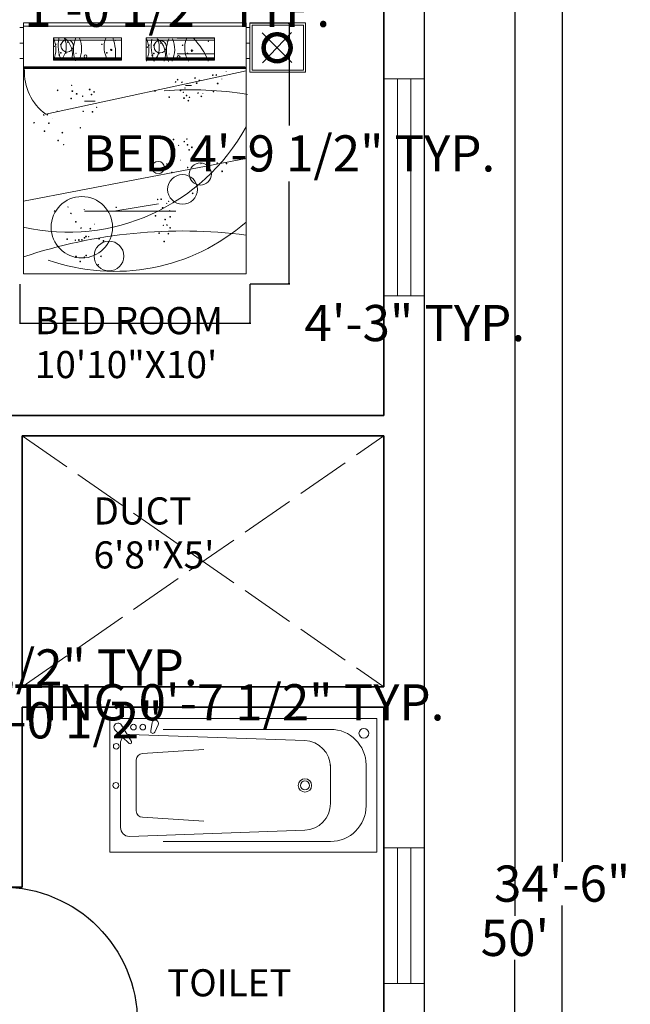
# Model space of a CAD drawing. Units: inches. Extents: x -11 to 443, y 65 to 743.
# Tile 9 of 10: x 243 to 378, y 392 to 610. Entities that reach past the tile are written whole.
import ezdxf

# ---------------------------------------------------------------- set-up
doc = ezdxf.new("R2010")
doc.units = ezdxf.units.IN
doc.header["$MEASUREMENT"] = 0
doc.linetypes.add('ACAD_ISO02W100', pattern=[15, 12, -3])
for name, color, linetype, lineweight in [('A-ANNO-DIMS', 2, 'Continuous', 18), ('A-AREA-IDEN', 2, 'Continuous', 18), ('A-DOOR', 4, 'Continuous', 25), ('A-FLOR-FIXT', 8, 'Continuous', 18), ('A-FLOR-VOID', 8, 'ACAD_ISO02W100', 13), ('A-FURN-PATT', 8, 'Continuous', 9), ('A-GLAZ', 4, 'Continuous', 18), ('A-WALL', 7, 'Continuous', 35), ('C-PROP', 3, 'Continuous', 30), ('Furniture', 7, 'Continuous', 15)]:
    doc.layers.add(name, color=color, linetype=linetype, lineweight=lineweight)
doc.styles.get("Standard").update_dxf_attribs({"font": 'italic8.shx'})
doc.dimstyles.get("Standard").update_dxf_attribs({"dimtxt": 8, "dimasz": 0.18, "dimexe": 0.18, "dimexo": 0.0625, "dimgap": 0.09, "dimtad": 0, "dimtih": 1, "dimtoh": 1, "dimzin": 0, "dimdsep": 46, "dimlunit": 3, "dimtxsty": 'Standard', "dimblk": 'CLOSEDBLANK', "dimcen": 0.09, "dimclrd": 6, "dimclre": 5, "dimclrt": 4, "dimadec": 0, "dimazin": 0, "dimtfac": 1, "dimtofl": 0, "dimtmove": 0, "dimatfit": 3, "dimfxl": 1, "dimtolj": 1, "dimtzin": 0, "dimarcsym": 0})

# ---------------------------------------------------------------- blocks, each defined once
blk = doc.blocks.new('_ClosedBlank')
at = {"color": 0, "linetype": 'ByBlock', "lineweight": -2}
for p, q in [((-1, 0.167), (0, 0)), ((-1, 0.167), (-1, -0.167)), ((0, 0), (-1, -0.167))]:
    blk.add_line(p, q, dxfattribs=at)
blk = doc.blocks.new('*D6')
at = {"layer": 'A-ANNO-DIMS', "color": 0, "lineweight": -2, "transparency": 16777216}
for p, q in [((332.27, 706.92), (352.4, 706.92)), ((352.22, 706.74), (352.22, 411.77)), ((352.22, 107.1), (352.22, 402.07)), ((332.27, 106.92), (352.4, 106.92))]:
    blk.add_line(p, q, dxfattribs=at)
at = {"layer": 'Defpoints', "color": 0, "lineweight": 100, "transparency": 16777216}
for p in [(332.21, 706.92), (332.21, 106.92), (352.22, 106.92)]:
    blk.add_point(p, dxfattribs=at)
at = {"layer": 'A-ANNO-DIMS', "color": 0, "lineweight": -2, "transparency": 16777216, "xscale": 0.18, "yscale": 0.18, "zscale": 0.18}
for p, rotation in [((352.22, 706.92), 90), ((352.22, 106.92), 270)]:
    blk.add_blockref('_ClosedBlank', p, dxfattribs=dict(at, rotation=rotation))
at = {"layer": 'A-ANNO-DIMS', "color": 0, "transparency": 16777216, "insert": (352.22, 406.92), "char_height": 8, "attachment_point": 5}
blk.add_mtext("\\A1;50'", dxfattribs=at)
blk = doc.blocks.new('DOOR-SWING-30')
for p, q in [((0, 30), (0, 0)), ((2, 29.93), (2, 0)), ((0, 0), (30, 0))]:
    blk.add_line(p, q)
blk.add_arc((0, 0), 30, 0, 90)
blk = doc.blocks.new('WIN-48x9')
for p, q in [((0, 48), (0, 0)), ((9, 48), (0, 48)), ((3, 0), (3, 48)), ((6, 0), (6, 48)), ((9, 0), (9, 48)), ((0, 0), (9, 0))]:
    blk.add_line(p, q)
blk = doc.blocks.new('BED-DOUBLE')
for p, q in [((0.82, 54.51), (0, 54.51)), ((50.12, 55.53), (0.82, 55.53)), ((0.82, 55.53), (0.82, 0)), ((50.12, 54.78), (0.82, 54.78)), ((50.12, 0), (50.12, 55.53)), ((50.12, 0), (50.12, 55.53)), ((50.95, 54.51), (50.12, 54.51)), ((0.82, 51.08), (0, 51.08)), ((7.45, 52.2), (7.45, 47.27)), ((22.51, 52.2), (7.45, 52.2)), ((7.45, 51.71), (22.51, 51.71)), ((22.51, 47.27), (22.51, 52.2)), ((43.08, 52.21), (28.01, 52.21)), ((28.01, 52.21), (28.01, 47.28)), ((28.01, 51.71), (43.1, 51.71)), ((43.08, 52.14), (34.85, 52.14)), ((43.08, 47.28), (43.08, 52.21)), ((50.95, 51.08), (50.12, 51.08)), ((43.08, 48.66), (34.85, 48.66)), ((0.82, 47.66), (0, 47.66)), ((0.82, 45.79), (49.9, 45.79)), ((7.45, 47.77), (22.51, 47.77)), ((7.45, 47.56), (22.51, 47.56)), ((7.45, 47.35), (22.51, 47.35)), ((7.45, 47.27), (22.51, 47.27)), ((28.01, 47.77), (43.1, 47.77)), ((28.01, 47.56), (43.1, 47.56)), ((28.01, 47.35), (43.1, 47.35)), ((28.01, 47.28), (43.08, 47.28)), ((50.95, 47.66), (50.12, 47.66)), ((0.81, 45.69), (50.11, 45.69)), ((0.81, 45.48), (50.11, 45.48)), ((5.76, 35.31), (50.13, 44.94)), ((38, 41.71), (36.72, 41.71)), ((16.71, 38.23), (14.33, 38.23)), ((0.81, 16.07), (50.11, 25.52)), ((30.69, 15.53), (20.82, 13.88)), ((34.54, 13.88), (14.33, 13.88)), ((0.82, 0), (50.12, 0)), ((0.82, 0), (50.12, 0))]:
    blk.add_line(p, q)
for centre, radius in [((7.67, 50.33), 0.0548), ((7.99, 50.77), 0.0548), ((9.09, 50.77), 0.0548), ((10.51, 50.44), 1.37), ((10.62, 51.21), 0.0274), ((10.95, 51.64), 0.0274), ((12.05, 51.64), 0.0274), ((12.05, 50.88), 0.0274), ((18.18, 50.77), 0.0548), ((21.14, 51.64), 0.0274), ((28.25, 50.16), 0.0548), ((28.58, 50.6), 0.0548), ((29.68, 50.6), 0.0548), ((31.1, 50.27), 1.37), ((31.21, 51.03), 0.0274), ((31.53, 51.47), 0.0274), ((32.63, 51.47), 0.0274), ((32.63, 50.71), 0.0274), ((36.03, 50.6), 0.0548), ((41.72, 51.47), 0.0274), ((8.76, 48.47), 0.0822), ((9.09, 48.91), 0.0822), ((10.19, 48.91), 0.0822), ((12.48, 48.8), 0.0274), ((14.56, 48.14), 0.329), ((19.27, 48.91), 0.0822), ((20.26, 49.56), 0.164), ((29.35, 48.3), 0.0822), ((29.67, 48.74), 0.0822), ((30.77, 48.74), 0.0822), ((33.07, 48.63), 0.0274), ((35.15, 47.97), 0.329), ((37.12, 48.74), 0.0822), ((38.11, 49.39), 0.164), ((41.53, 45.6), 0.0822), ((42.72, 43.97), 0.0548), ((43.5, 44.01), 0.0822), ((45.68, 44.84), 0.0274), ((11.51, 41.72), 0.0548), ((34.49, 42.48), 0.0548), ((34.94, 42.97), 0.0822), ((35.9, 42.4), 0.0822), ((38.78, 43.35), 0.0822), ((39.16, 42.2), 0.0822), ((39.74, 42.78), 0.0822), ((43.81, 42.11), 0.0822), ((44.72, 43.1), 0.0274), ((8.39, 40.62), 0.0822), ((11.65, 40.43), 0.0822), ((12.61, 39.86), 0.0822), ((13.92, 39.31), 0.0548), ((15.49, 40.82), 0.0822), ((15.87, 39.67), 0.0822), ((16.44, 40.24), 0.0822), ((29.94, 40.51), 0.0822), ((35.59, 40.62), 0.0822), ((36.22, 40.19), 0.0548), ((36.59, 41.14), 0.0274), ((36.93, 39.48), 0.0822), ((39.48, 40), 0.0548), ((40.19, 39.28), 0.0822), ((40.52, 39.93), 0.0274), ((42.86, 40.37), 0.0822), ((11.37, 38.79), 0.0822), ((33.1, 39.09), 0.0822), ((36.35, 38.9), 0.0822), ((37.31, 38.33), 0.0822), ((37.56, 39.06), 0.0548), ((5.33, 35.19), 0.0548), ((6.11, 35.23), 0.0822), ((8.29, 36.06), 0.0274), ((14.06, 35.98), 0.0548), ((16.11, 35.86), 0.0822), ((17.02, 36.86), 0.0274), ((3.2, 33.44), 0.0548), ((6.43, 33.33), 0.0822), ((7.34, 34.32), 0.0274), ((5.48, 31.58), 0.0822), ((9.44, 31.26), 0.0822), ((13.43, 32.33), 0.0548), ((8.49, 29.52), 0.0822), ((9.72, 28.61), 0.0274), ((33.86, 28.77), 0.0822), ((34.05, 29.73), 0.0822), ((35.15, 28.44), 0.0274), ((36.41, 29.29), 0.0548), ((36.99, 29.87), 0.0548), ((37.12, 28.58), 0.0822), ((34.24, 27.62), 0.0822), ((37.5, 27.43), 0.0822), ((38.08, 28.01), 0.0822), ((30.66, 23.53), 1.37), ((32.57, 24.29), 0.0548), ((33.81, 25.44), 0.0274), ((35.53, 25.17), 0.0274), ((39.97, 22.1), 2.46), ((40.13, 24.42), 0.0274), ((43.71, 24.56), 0.0548), ((45.75, 24.45), 0.0822), ((36.03, 18.71), 3.29), ((33.67, 22.43), 0.0822), ((37.18, 23.55), 0.0548), ((44.8, 22.7), 0.0822), ((38.27, 17.83), 0.0822), ((13.75, 10.33), 6.79), ((30.53, 16.48), 0.0548), ((31.31, 16.52), 0.0822), ((32.54, 15.61), 0.0274), ((32.96, 16.06), 0.0548), ((7.71, 13.94), 0.0548), ((10.67, 14.82), 0.0274), ((11.32, 13.38), 0.0548), ((14.28, 14.25), 0.0274), ((21.36, 14.74), 0.0548), ((31.63, 14.62), 0.0822), ((33.15, 13.95), 0.0548), ((12.42, 11.52), 0.0822), ((16.54, 11.02), 0.0274), ((30.03, 12.86), 0.0822), ((32.19, 12.04), 0.0548), ((32.58, 10.82), 0.0822), ((33.29, 12.66), 0.0822), ((13.59, 10.14), 0.0548), ((15.63, 10.02), 0.0822), ((30.85, 9.03), 0.0548), ((31.8, 10.77), 0.0548), ((32.9, 8.91), 0.0822), ((33.29, 10.18), 0.0822), ((10.5, 7.72), 0.0822), ((12.32, 7.47), 0.0548), ((13.09, 7.51), 0.0822), ((13.76, 7.53), 0.0822), ((14.33, 8.01), 0.0822), ((14.68, 8.28), 0.0822), ((15.27, 8.25), 0.0274), ((19.76, 3.97), 3.29), ((17.59, 7.82), 0.0822), ((18.55, 7.34), 0.0822), ((31.95, 7.17), 0.0822), ((12.46, 3.87), 0.0822), ((13.41, 2.75), 0.0822), ((14.32, 3.74), 0.0274), ((14.72, 4.1), 0.0822), ((17.98, 3.91), 0.0822), ((17.39, 2.05), 0.0548)]:
    blk.add_circle(centre, radius)
for centre, radius, start, end in [((10.49, 48.64), 10.74, 352.6491, 19.9229), ((2.24, 49.73), 5.76, 334.6876, 25.3124), ((18.3, 50.59), 9.77, 171.2054, 199.8717), ((5.97, 50.26), 4.34, 316.473, 26.5351), ((7.41, 48.73), 4.24, 339.7755, 54.8367), ((18.16, 49.62), 6.28, 155.7867, 203.0598), ((7.63, 49.85), 6.08, 334.8533, 22.5945), ((24.13, 50.16), 5.46, 158.1924, 212.0094), ((22.83, 49.56), 5.76, 334.6876, 25.3124), ((38.89, 50.42), 9.77, 171.2054, 199.8717), ((26.55, 50.09), 4.34, 316.473, 26.5351), ((28, 48.56), 4.24, 339.7755, 54.8367), ((38.74, 49.45), 6.28, 155.7867, 203.0598), ((28.22, 49.68), 6.08, 334.8533, 22.5945), ((41.97, 49.99), 5.46, 158.1924, 212.0094), ((27.71, 41.52), 15.09, 21.7027, 44.6945), ((12.77, 44.72), 11.73, 177.3999, 233.2824), ((37.95, -36.79), 77.52, 80.7462, 94.4176), ((10.65, 54.27), 45.03, 257.3742, 331.1748), ((20.99, 44.94), 44.36, 250.6919, 311.0239), ((35.98, -101.04), 110.55, 82.6585, 108.5509)]:
    blk.add_arc(centre, radius, start, end)
blk = doc.blocks.new('NIGHTSTAND-LAMP')
for p, q in [((0, 10.9), (0, 0)), ((12.32, 10.9), (0, 10.9)), ((12.32, 0), (12.32, 10.9)), ((0.49, 10.41), (0.49, 0.49)), ((11.83, 10.41), (0.49, 10.41)), ((2.81, 2.1), (9.21, 8.77)), ((11.83, 0.49), (11.83, 10.41)), ((2.74, 8.7), (9.27, 2.17)), ((0.49, 0.49), (11.83, 0.49)), ((0, 0), (12.32, 0))]:
    blk.add_line(p, q)
for radius in [3.39, 2.6]:
    blk.add_circle((6.01, 5.43), radius)
blk = doc.blocks.new('*D24')
at = {"layer": 'A-ANNO-DIMS', "color": 5, "lineweight": -2, "transparency": 16777216}
for p, q in [((293.66, 609.27), (302.43, 609.27)), ((293.66, 551.54), (302.43, 551.54))]:
    blk.add_line(p, q, dxfattribs=at)
at = {"layer": 'A-ANNO-DIMS', "color": 6, "lineweight": -2, "transparency": 16777216}
for p, q in [((302.25, 609.09), (302.25, 586.59)), ((302.25, 551.72), (302.25, 574.22))]:
    blk.add_line(p, q, dxfattribs=at)
at = {"layer": 'Defpoints', "color": 0, "lineweight": 100, "transparency": 16777216}
for p in [(293.59, 609.27), (302.25, 609.27), (293.59, 551.54)]:
    blk.add_point(p, dxfattribs=at)
at = {"layer": 'A-ANNO-DIMS', "color": 6, "lineweight": -2, "transparency": 16777216, "xscale": 0.18, "yscale": 0.18, "zscale": 0.18}
for p, rotation in [((302.25, 609.27), 90), ((302.25, 551.54), 270)]:
    blk.add_blockref('_ClosedBlank', p, dxfattribs=dict(at, rotation=rotation))
at = {"layer": 'A-ANNO-DIMS', "color": 4, "transparency": 16777216, "insert": (302.25, 580.41), "char_height": 8, "attachment_point": 5}
blk.add_mtext('\\A1;BED 4\'-9 1/2" TYP.', dxfattribs=at)
blk = doc.blocks.new('*D25')
at = {"layer": 'A-ANNO-DIMS', "color": 5, "lineweight": -2, "transparency": 16777216}
for p, q in [((242.65, 551.48), (242.65, 542.71)), ((293.59, 551.48), (293.59, 542.71))]:
    blk.add_line(p, q, dxfattribs=at)
at = {"layer": 'A-ANNO-DIMS', "color": 6, "lineweight": -2, "transparency": 16777216}
for p, q in [((242.83, 542.89), (293.41, 542.89)), ((293.59, 542.89), (293.77, 542.89))]:
    blk.add_line(p, q, dxfattribs=at)
at = {"layer": 'Defpoints', "color": 0, "lineweight": 100, "transparency": 16777216}
for p in [(242.65, 551.54), (293.59, 551.54), (293.59, 542.89)]:
    blk.add_point(p, dxfattribs=at)
at = {"layer": 'A-ANNO-DIMS', "color": 6, "lineweight": -2, "transparency": 16777216, "xscale": 0.18, "yscale": 0.18, "zscale": 0.18, "rotation": 180}
blk.add_blockref('_ClosedBlank', (242.65, 542.89), dxfattribs=at)
at = {"layer": 'A-ANNO-DIMS', "color": 6, "lineweight": -2, "transparency": 16777216, "xscale": 0.18, "yscale": 0.18, "zscale": 0.18}
blk.add_blockref('_ClosedBlank', (293.59, 542.89), dxfattribs=at)
at = {"layer": 'A-ANNO-DIMS', "color": 4, "transparency": 16777216, "insert": (330.05, 542.89), "char_height": 8, "attachment_point": 5}
blk.add_mtext('\\A1;4\'-3" TYP.', dxfattribs=at)
blk = doc.blocks.new('*D26')
at = {"layer": 'A-ANNO-DIMS', "color": 5, "lineweight": -2, "transparency": 16777216}
for p, q in [((133.01, 610.6), (133.01, 612.57)), ((145.34, 610.6), (145.34, 612.57))]:
    blk.add_line(p, q, dxfattribs=at)
at = {"layer": 'A-ANNO-DIMS', "color": 6, "lineweight": -2, "transparency": 16777216}
for p, q in [((133.19, 612.39), (145.16, 612.39)), ((145.34, 612.39), (145.52, 612.39))]:
    blk.add_line(p, q, dxfattribs=at)
at = {"layer": 'Defpoints', "color": 0, "lineweight": 100, "transparency": 16777216}
for p in [(145.34, 612.39), (133.01, 610.54), (145.34, 610.54)]:
    blk.add_point(p, dxfattribs=at)
at = {"layer": 'A-ANNO-DIMS', "color": 6, "lineweight": -2, "transparency": 16777216, "xscale": 0.18, "yscale": 0.18, "zscale": 0.18, "rotation": 180}
blk.add_blockref('_ClosedBlank', (133.01, 612.39), dxfattribs=at)
at = {"layer": 'A-ANNO-DIMS', "color": 6, "lineweight": -2, "transparency": 16777216, "xscale": 0.18, "yscale": 0.18, "zscale": 0.18}
blk.add_blockref('_ClosedBlank', (145.34, 612.39), dxfattribs=at)
at = {"layer": 'A-ANNO-DIMS', "color": 4, "transparency": 16777216, "insert": (242.18, 612.39), "char_height": 8, "attachment_point": 5}
blk.add_mtext('\\A1;NIGHTSTAND 1\'-0 1/2" TYP.', dxfattribs=at)
blk = doc.blocks.new('*D30')
at = {"layer": 'A-ANNO-DIMS', "color": 5, "lineweight": -2, "transparency": 16777216}
for p, q in [((187.91, 460.07), (187.91, 458.84)), ((195.36, 460.07), (195.36, 458.84))]:
    blk.add_line(p, q, dxfattribs=at)
at = {"layer": 'A-ANNO-DIMS', "color": 6, "lineweight": -2, "transparency": 16777216}
for p, q in [((188.09, 459.02), (195.18, 459.02)), ((195.36, 459.02), (195.54, 459.02))]:
    blk.add_line(p, q, dxfattribs=at)
at = {"layer": 'Defpoints', "color": 0, "lineweight": 100, "transparency": 16777216}
for p in [(187.91, 460.14), (195.36, 460.14), (195.36, 459.02)]:
    blk.add_point(p, dxfattribs=at)
at = {"layer": 'A-ANNO-DIMS', "color": 6, "lineweight": -2, "transparency": 16777216, "xscale": 0.18, "yscale": 0.18, "zscale": 0.18, "rotation": 180}
blk.add_blockref('_ClosedBlank', (187.91, 459.02), dxfattribs=at)
at = {"layer": 'A-ANNO-DIMS', "color": 6, "lineweight": -2, "transparency": 16777216, "xscale": 0.18, "yscale": 0.18, "zscale": 0.18}
blk.add_blockref('_ClosedBlank', (195.36, 459.02), dxfattribs=at)
at = {"layer": 'A-ANNO-DIMS', "color": 4, "transparency": 16777216, "insert": (279.25, 459.02), "char_height": 8, "attachment_point": 5}
blk.add_mtext('\\A1;SETTING 0\'-7 1/2" TYP.', dxfattribs=at)
blk = doc.blocks.new('*D31')
at = {"layer": 'A-ANNO-DIMS', "color": 5, "lineweight": -2, "transparency": 16777216}
for p, q in [((195.43, 466.55), (196.66, 466.55)), ((195.43, 460.14), (196.66, 460.14))]:
    blk.add_line(p, q, dxfattribs=at)
at = {"layer": 'A-ANNO-DIMS', "color": 6, "lineweight": -2, "transparency": 16777216}
for p, q in [((196.48, 466.55), (196.48, 466.73)), ((196.48, 466.73), (196.66, 466.73)), ((196.48, 460.32), (196.48, 466.37))]:
    blk.add_line(p, q, dxfattribs=at)
at = {"layer": 'Defpoints', "color": 0, "lineweight": 100, "transparency": 16777216}
for p in [(195.36, 466.55), (196.48, 466.55), (195.36, 460.14)]:
    blk.add_point(p, dxfattribs=at)
at = {"layer": 'A-ANNO-DIMS', "color": 6, "lineweight": -2, "transparency": 16777216, "xscale": 0.18, "yscale": 0.18, "zscale": 0.18}
for p, rotation in [((196.48, 466.55), 90), ((196.48, 460.14), 270)]:
    blk.add_blockref('_ClosedBlank', p, dxfattribs=dict(at, rotation=rotation))
at = {"layer": 'A-ANNO-DIMS', "color": 4, "transparency": 16777216, "insert": (248.18, 466.73), "char_height": 8, "attachment_point": 5}
blk.add_mtext('\\A1;0\'-6 1/2" TYP.', dxfattribs=at)
blk = doc.blocks.new('*D36')
at = {"layer": 'A-ANNO-DIMS', "color": 5, "lineweight": -2, "transparency": 16777216}
for p, q in [((323.27, 625.92), (362.85, 625.92)), ((323.27, 211.92), (362.85, 211.92))]:
    blk.add_line(p, q, dxfattribs=at)
at = {"layer": 'A-ANNO-DIMS', "color": 6, "lineweight": -2, "transparency": 16777216}
for p, q in [((362.67, 625.74), (362.67, 423.77)), ((362.67, 212.1), (362.67, 414.07))]:
    blk.add_line(p, q, dxfattribs=at)
at = {"layer": 'Defpoints', "color": 0, "lineweight": 100, "transparency": 16777216}
for p in [(323.21, 625.92), (362.67, 625.92), (323.21, 211.92)]:
    blk.add_point(p, dxfattribs=at)
at = {"layer": 'A-ANNO-DIMS', "color": 6, "lineweight": -2, "transparency": 16777216, "xscale": 0.18, "yscale": 0.18, "zscale": 0.18}
for p, rotation in [((362.67, 625.92), 90), ((362.67, 211.92), 270)]:
    blk.add_blockref('_ClosedBlank', p, dxfattribs=dict(at, rotation=rotation))
at = {"layer": 'A-ANNO-DIMS', "color": 4, "transparency": 16777216, "insert": (362.67, 418.92), "char_height": 8, "attachment_point": 5}
blk.add_mtext('\\A1;34\'-6"', dxfattribs=at)
blk = doc.blocks.new('*D41')
at = {"layer": 'A-ANNO-DIMS', "color": 5, "lineweight": -2, "transparency": 16777216}
for p, q in [((191.4, 454.94), (191.4, 455.12)), ((191.31, 455.03), (191.49, 455.03))]:
    blk.add_line(p, q, dxfattribs=at)
at = {"layer": 'A-ANNO-DIMS', "color": 6, "lineweight": -2, "transparency": 16777216}
blk.add_line((210.85, 455.03), (203.74, 455.03), dxfattribs=at)
at = {"layer": 'Defpoints', "color": 0, "lineweight": 100, "transparency": 16777216}
for p in [(179.23, 455.03), (203.56, 455.03)]:
    blk.add_point(p, dxfattribs=at)
at = {"layer": 'A-ANNO-DIMS', "color": 6, "lineweight": -2, "transparency": 16777216, "xscale": 0.18, "yscale": 0.18, "zscale": 0.18, "rotation": 179.9993686908669}
blk.add_blockref('_ClosedBlank', (203.56, 455.03), dxfattribs=at)
at = {"layer": 'A-ANNO-DIMS', "color": 4, "transparency": 16777216, "insert": (247.32, 455.03), "char_height": 8, "attachment_point": 5}
blk.add_mtext('\\A1;∅2\'-0 1/2"', dxfattribs=at)

msp = doc.modelspace()

# ---------------------------------------------------------------- hatches: boundary and pattern name
at = {"layer": 'A-FURN-PATT'}
h = msp.add_hatch(dxfattribs=at)
h.set_pattern_fill('ANSI37', color=256, scale=0.6260848, angle=45, style=0)
h.paths.add_polyline_path([(302.989, 603.779), (302.987, 603.912), (302.979, 604.045), (302.966, 604.177), (302.947, 604.309), (302.924, 604.44), (302.896, 604.57), (302.862, 604.698), (302.823, 604.826), (302.78, 604.951), (302.731, 605.075), (302.678, 605.197), (302.62, 605.317), (302.557, 605.434), (302.49, 605.549), (302.418, 605.661), (302.342, 605.77), (302.262, 605.876), (302.177, 605.979), (302.089, 606.079), (301.997, 606.175), (301.901, 606.267), (301.801, 606.355), (301.699, 606.44), (301.592, 606.52), (301.483, 606.596), (301.371, 606.668), (301.256, 606.735), (301.139, 606.798), (301.019, 606.856), (300.897, 606.909), (300.774, 606.958), (300.648, 607.001), (300.521, 607.04), (300.392, 607.073), (300.262, 607.102), (300.131, 607.125), (299.999, 607.144), (299.867, 607.157), (299.734, 607.164), (299.601, 607.167), (299.468, 607.164), (299.335, 607.157), (299.203, 607.144), (299.071, 607.125), (298.94, 607.102), (298.81, 607.073), (298.681, 607.04), (298.554, 607.001), (298.428, 606.958), (298.304, 606.909), (298.182, 606.856), (298.063, 606.798), (297.945, 606.735), (297.83, 606.668), (297.718, 606.596), (297.609, 606.52), (297.503, 606.44), (297.4, 606.355), (297.301, 606.267), (297.205, 606.175), (297.113, 606.079), (297.024, 605.979), (296.94, 605.876), (296.86, 605.77), (296.784, 605.661), (296.712, 605.549), (296.645, 605.434), (296.582, 605.317), (296.524, 605.197), (296.47, 605.075), (296.422, 604.951), (296.378, 604.826), (296.34, 604.698), (296.306, 604.57), (296.278, 604.44), (296.254, 604.309), (296.236, 604.177), (296.223, 604.045), (296.215, 603.912), (296.213, 603.779), (296.215, 603.646), (296.223, 603.513), (296.236, 603.38), (296.254, 603.249), (296.278, 603.118), (296.306, 602.988), (296.34, 602.859), (296.378, 602.732), (296.422, 602.606), (296.47, 602.482), (296.524, 602.36), (296.582, 602.24), (296.645, 602.123), (296.712, 602.008), (296.784, 601.896), (296.86, 601.787), (296.94, 601.681), (297.024, 601.578), (297.113, 601.479), (297.205, 601.383), (297.301, 601.291), (297.4, 601.202), (297.503, 601.118), (297.609, 601.038), (297.718, 600.961), (297.83, 600.89), (297.945, 600.822), (298.063, 600.76), (298.182, 600.702), (298.304, 600.648), (298.428, 600.6), (298.554, 600.556), (298.681, 600.518), (298.81, 600.484), (298.94, 600.456), (299.071, 600.432), (299.203, 600.414), (299.335, 600.401), (299.468, 600.393), (299.601, 600.39), (299.734, 600.393), (299.867, 600.401), (299.999, 600.414), (300.131, 600.432), (300.262, 600.456), (300.392, 600.484), (300.521, 600.518), (300.648, 600.556), (300.774, 600.6), (300.897, 600.648), (301.019, 600.702), (301.139, 600.76), (301.256, 600.822), (301.371, 600.89), (301.483, 600.961), (301.592, 601.038), (301.699, 601.118), (301.801, 601.202), (301.901, 601.291), (301.997, 601.383), (302.089, 601.479), (302.177, 601.578), (302.262, 601.681), (302.342, 601.787), (302.418, 601.896), (302.49, 602.008), (302.557, 602.123), (302.62, 602.24), (302.678, 602.36), (302.731, 602.482), (302.78, 602.606), (302.823, 602.732), (302.862, 602.859), (302.896, 602.988), (302.924, 603.118), (302.947, 603.249), (302.966, 603.38), (302.979, 603.513), (302.987, 603.646)])
h.paths.add_polyline_path([(302.206, 603.779), (302.204, 603.676), (302.198, 603.574), (302.188, 603.473), (302.174, 603.371), (302.156, 603.271), (302.134, 603.171), (302.108, 603.072), (302.078, 602.974), (302.045, 602.877), (302.007, 602.782), (301.966, 602.688), (301.922, 602.596), (301.874, 602.506), (301.822, 602.418), (301.767, 602.332), (301.708, 602.248), (301.646, 602.166), (301.582, 602.087), (301.514, 602.011), (301.443, 601.937), (301.369, 601.866), (301.293, 601.798), (301.213, 601.733), (301.132, 601.671), (301.048, 601.613), (300.962, 601.558), (300.874, 601.506), (300.783, 601.458), (300.691, 601.413), (300.598, 601.372), (300.502, 601.335), (300.406, 601.301), (300.308, 601.272), (300.209, 601.246), (300.109, 601.224), (300.008, 601.206), (299.907, 601.192), (299.805, 601.182), (299.703, 601.176), (299.601, 601.174), (299.499, 601.176), (299.396, 601.182), (299.295, 601.192), (299.193, 601.206), (299.093, 601.224), (298.993, 601.246), (298.894, 601.272), (298.796, 601.301), (298.699, 601.335), (298.604, 601.372), (298.51, 601.413), (298.418, 601.458), (298.328, 601.506), (298.24, 601.558), (298.154, 601.613), (298.07, 601.671), (297.988, 601.733), (297.909, 601.798), (297.833, 601.866), (297.759, 601.937), (297.688, 602.011), (297.62, 602.087), (297.555, 602.166), (297.494, 602.248), (297.435, 602.332), (297.38, 602.418), (297.328, 602.506), (297.28, 602.596), (297.235, 602.688), (297.194, 602.782), (297.157, 602.877), (297.124, 602.974), (297.094, 603.072), (297.068, 603.171), (297.046, 603.271), (297.028, 603.371), (297.014, 603.473), (297.004, 603.574), (296.998, 603.676), (296.996, 603.779), (296.998, 603.881), (297.004, 603.983), (297.014, 604.085), (297.028, 604.186), (297.046, 604.287), (297.068, 604.387), (297.094, 604.486), (297.124, 604.584), (297.157, 604.68), (297.194, 604.776), (297.235, 604.869), (297.28, 604.961), (297.328, 605.051), (297.38, 605.14), (297.435, 605.226), (297.494, 605.31), (297.555, 605.391), (297.62, 605.47), (297.688, 605.547), (297.759, 605.621), (297.833, 605.691), (297.909, 605.759), (297.988, 605.824), (298.07, 605.886), (298.154, 605.945), (298.24, 606), (298.328, 606.051), (298.418, 606.1), (298.51, 606.144), (298.604, 606.185), (298.699, 606.223), (298.796, 606.256), (298.894, 606.286), (298.993, 606.312), (299.093, 606.333), (299.193, 606.351), (299.295, 606.365), (299.396, 606.376), (299.499, 606.382), (299.601, 606.384), (299.703, 606.382), (299.805, 606.376), (299.907, 606.365), (300.008, 606.351), (300.109, 606.333), (300.209, 606.312), (300.308, 606.286), (300.406, 606.256), (300.502, 606.223), (300.598, 606.185), (300.691, 606.144), (300.783, 606.1), (300.874, 606.051), (300.962, 606), (301.048, 605.945), (301.132, 605.886), (301.213, 605.824), (301.293, 605.759), (301.369, 605.691), (301.443, 605.621), (301.514, 605.547), (301.582, 605.47), (301.646, 605.391), (301.708, 605.31), (301.767, 605.226), (301.822, 605.14), (301.874, 605.051), (301.922, 604.961), (301.966, 604.869), (302.007, 604.776), (302.045, 604.68), (302.078, 604.584), (302.108, 604.486), (302.134, 604.387), (302.156, 604.287), (302.174, 604.186), (302.188, 604.085), (302.198, 603.983), (302.204, 603.881)], flags=0)

# ---------------------------------------------------------------- linework, layer by layer
at = {"layer": 'A-FLOR-FIXT'}
for p, q in [((321.647, 455.401), (262.592, 455.401)), ((262.592, 455.401), (262.592, 425.874)), ((321.647, 425.874), (321.647, 455.401)), ((267.374, 450.325), (265.186, 453.955)), ((271.942, 454.519), (271.636, 452.692)), ((272.529, 452.413), (273.292, 454.034)), ((311.411, 453.039), (274.403, 453.039)), ((263.744, 452.888), (266.889, 449.933)), ((266.923, 451.912), (305.712, 450.556)), ((264.954, 449.944), (264.954, 431.331)), ((269.823, 447.665), (283.355, 448.561)), ((268.445, 446.287), (268.445, 434.988)), ((311.411, 436.62), (311.411, 445.165)), ((319.285, 436.11), (319.285, 445.165)), ((269.823, 433.61), (283.355, 432.714)), ((266.923, 429.363), (305.712, 430.718)), ((274.403, 428.236), (311.411, 428.236)), ((262.592, 425.874), (321.647, 425.874))]:
    msp.add_line(p, q, dxfattribs=at)
for centre, radius in [((267.818, 453.531), 0.628), ((269.883, 453.531), 0.628), ((318.797, 452.162), 1.086), ((264.013, 449.286), 0.628), ((305.767, 440.637), 1.476), ((263.934, 440.637), 0.656), ((305.767, 440.637), 0.984)]:
    msp.add_circle(centre, radius, dxfattribs=at)
for centre, radius, start, end in [((264.404, 453.504), 0.903, 29.98081, 223.02252), ((272.644, 454.354), 0.722, 333.70215, 166.74386), ((311.411, 445.165), 7.874, 0, 90), ((266.923, 449.944), 1.968, 137.68629, 180), ((266.923, 449.944), 1.968, 137.68629, 180), ((266.923, 449.944), 1.968, 90, 103.84203), ((266.923, 449.944), 1.968, 90, 103.84203), ((272.102, 452.614), 0.472, 170.49628, 334.80018), ((267.105, 450.162), 0.315, 226.77494, 31.07884), ((267.105, 450.162), 0.315, 226.77494, 31.07884), ((305.506, 444.655), 5.905, 0, 87.99837), ((269.823, 446.287), 1.378, 90, 180), ((305.506, 436.62), 5.905, 272.00163, 0), ((311.411, 436.11), 7.874, 270, 0), ((269.823, 434.988), 1.378, 180, 270), ((266.923, 431.331), 1.968, 180, 270)]:
    msp.add_arc(centre, radius, start, end, dxfattribs=at)
at = {"layer": 'A-FLOR-VOID'}
for p, q in [((243.209, 462.42), (323.209, 517.92)), ((243.209, 517.92), (323.209, 462.42))]:
    msp.add_line(p, q, dxfattribs=at)
at = {"layer": 'A-GLAZ'}
for p, q in [((323.209, 396.826), (323.209, 426.826)), ((323.209, 426.826), (332.209, 426.826)), ((326.209, 426.826), (326.209, 396.826)), ((329.209, 426.826), (329.209, 396.826)), ((332.209, 426.826), (332.209, 396.826)), ((332.209, 396.826), (323.209, 396.826))]:
    msp.add_line(p, q, dxfattribs=at)
at = {"layer": 'A-WALL'}
for p, q in [((323.209, 522.42), (323.209, 616.92)), ((236.859, 522.42), (323.209, 522.42)), ((243.209, 517.92), (323.209, 517.92)), ((243.209, 462.42), (243.209, 517.92)), ((323.209, 462.42), (323.209, 517.92)), ((243.209, 462.42), (323.209, 462.42)), ((243.209, 457.92), (323.209, 457.92)), ((243.209, 418.17), (243.209, 457.92)), ((323.209, 378.42), (323.209, 457.92)), ((243.209, 418.17), (238.709, 418.17))]:
    msp.add_line(p, q, dxfattribs=at)
at = {"layer": 'C-PROP'}
msp.add_lwpolyline([(44.209, 106.92), (332.209, 106.92), (332.209, 706.92), (44.209, 706.92)], close=True, dxfattribs=at)

# ---------------------------------------------------------------- block references
at = {"layer": 'A-DOOR', "extrusion": (0, 0, -1), "zscale": -1, "rotation": 90.00000000000003}
msp.add_blockref('DOOR-SWING-30', (-238.709, 388.169), dxfattribs=at)
at = {"layer": 'A-GLAZ'}
msp.add_blockref('WIN-48x9', (323.209, 548.882), dxfattribs=at)
at = {"layer": 'Furniture'}
for name, p in [('BED-DOUBLE', (242.648, 553.738)), ('NIGHTSTAND-LAMP', (293.594, 598.345))]:
    msp.add_blockref(name, p, dxfattribs=at)

# ---------------------------------------------------------------- texts
at = {"layer": 'A-AREA-IDEN'}
for s, p in [('BED ROOM', (245.989, 540.418)), ('10\'10"X10\'', (245.989, 530.704)), ('DUCT', (258.989, 498.336)), ('6\'8"X5\'', (258.989, 488.622)), ('TOILET', (275.264, 393.986))]:
    msp.add_text(s, height=6, dxfattribs=at).set_placement(p)

# ---------------------------------------------------------------- dimensions: what is measured, and where the dimension line sits
at = {"layer": 'A-ANNO-DIMS'}
for base, p1, p2, override, picture, middle in [((352.221, 106.92), (332.209, 706.92), (332.209, 106.92), {"dimclrd": 0, "dimclre": 0, "dimclrt": 0}, '*D6', (352.221, 406.92)), ((362.669, 625.92), (323.209, 211.92), (323.209, 625.92), {"dimdec": 1, "dimlfac": 1, "dimrnd": 0, "dimzin": 1, "dimdsep": 46, "dimlunit": 4, "dimfrac": 2}, '*D36', (362.669, 418.92))]:
    dim = msp.add_linear_dim(base=base, p1=p1, p2=p2, angle=90, dimstyle='Standard', override=override, dxfattribs=at)
    dim.commit()
    dim.dimension.update_dxf_attribs({"geometry": picture, "text_midpoint": middle})
for base, p1, p2, text, picture, middle in [((145.337, 612.387), (133.013, 610.539), (145.337, 610.539), 'NIGHTSTAND <> TYP.', '*D26', (242.179, 612.387)), ((293.593, 542.886), (242.648, 551.544), (293.593, 551.544), '<> TYP.', '*D25', (330.054, 542.886)), ((195.365, 459.019), (187.912, 460.137), (195.365, 460.137), 'SETTING <> TYP.', '*D30', (279.254, 459.019))]:
    dim = msp.add_linear_dim(base=base, p1=p1, p2=p2, text=text, dimstyle='Standard', override={"dimdec": 1, "dimlfac": 1, "dimrnd": 0, "dimzin": 1, "dimdsep": 46, "dimlunit": 4, "dimfrac": 2}, dxfattribs=at)
    dim.commit()
    dim.dimension.update_dxf_attribs({"geometry": picture, "text_midpoint": middle})
for base, p1, p2, text, picture, middle in [((302.252, 609.267), (293.593, 551.544), (293.593, 609.267), 'BED <> TYP.', '*D24', (302.252, 580.406)), ((196.483, 466.551), (195.365, 460.137), (195.365, 466.551), '<> TYP.', '*D31', (248.181, 466.731))]:
    dim = msp.add_linear_dim(base=base, p1=p1, p2=p2, angle=90, text=text, dimstyle='Standard', override={"dimdec": 1, "dimlfac": 1, "dimrnd": 0, "dimzin": 1, "dimdsep": 46, "dimlunit": 4, "dimfrac": 2}, dxfattribs=at)
    dim.commit()
    dim.dimension.update_dxf_attribs({"geometry": picture, "text_midpoint": middle})
dim = msp.add_diameter_dim_2p(p1=(179.234, 455.031), p2=(203.557, 455.031), dimstyle='Standard', override={"dimdec": 1, "dimlfac": 1, "dimrnd": 0, "dimzin": 1, "dimdsep": 46, "dimlunit": 4, "dimfrac": 2}, dxfattribs=at)
dim.commit()
dim.dimension.update_dxf_attribs({"geometry": '*D41', "text_midpoint": (210.854, 455.031), "dimtype": 163})

doc.saveas('drawing.dxf')
